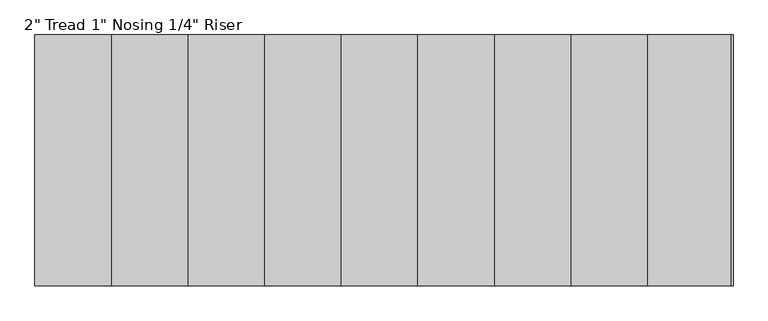
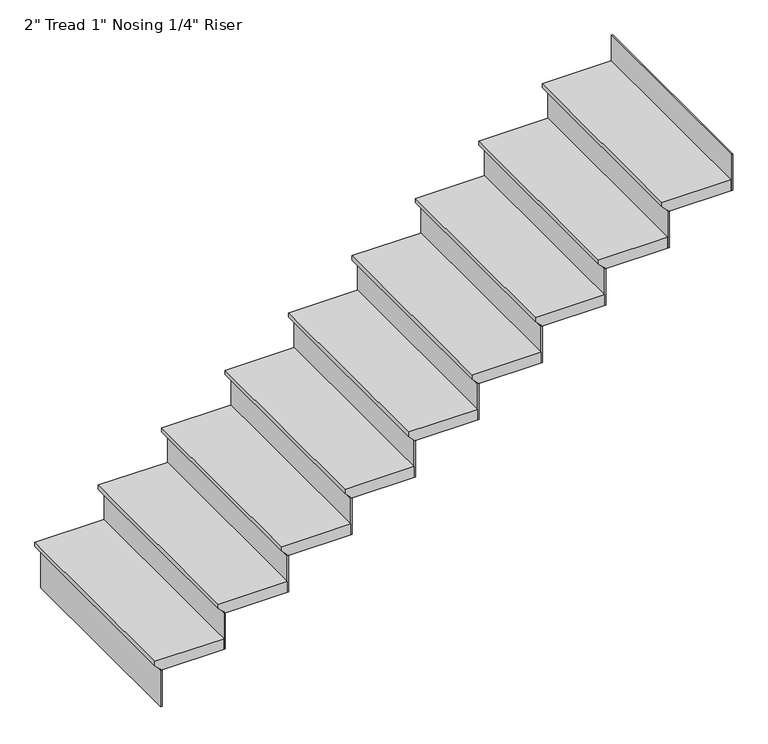
"""IFC4 building model written with IfcOpenShell, lengths in millimetres: stair flight geometry."""

from ifc_helpers import new_model, si_unit, frame, origin, place, context, project, spatial, polyline, outline, extrude, source, transform, mapped, element, save


def stair_flight_c7e5c723(model_context):
    return source(origin(), model_context, "Body", "SweptSolid", [
        extrude(outline(polyline([(4876.8, -14271.1777023), (4876.8, -14575.9777023), (4857.75, -14575.9777023), (4832.35, -14550.5777023), (4826.0, -14550.5777023), (4826.0, -14271.1777023), (4876.8, -14271.1777023)])), frame((0.0, 788.0679075, 0.0), z_axis=(0.0, 1.0, 0.0), x_axis=(0.0, 0.0, 1.0)), (0.0, 0.0, 1.0), 914.4),
        extrude(outline(polyline([(-14544.2277023, 788.0679075), (-14550.5777023, 788.0679075), (-14550.5777023, 1702.4679075), (-14544.2277023, 1702.4679075), (-14544.2277023, 788.0679075)])), frame((0.0, 0.0, 4656.6666667), z_axis=(0.0, 0.0, 1.0), x_axis=(1.0, 0.0, 0.0)), (0.0, 0.0, 1.0), 169.3333333),
        extrude(outline(polyline([(-14264.8277023, 788.0679075), (-14271.1777023, 788.0679075), (-14271.1777023, 1702.4679075), (-14264.8277023, 1702.4679075), (-14264.8277023, 788.0679075)])), frame((0.0, 0.0, 4826.0), z_axis=(0.0, 0.0, 1.0), x_axis=(1.0, 0.0, 0.0)), (0.0, 0.0, 1.0), 169.3333333),
        extrude(outline(polyline([(5046.1333333, -13991.7777023), (5046.1333333, -14296.5777023), (5027.0833333, -14296.5777023), (5001.6833333, -14271.1777023), (4995.3333333, -14271.1777023), (4995.3333333, -13991.7777023), (5046.1333333, -13991.7777023)])), frame((0.0, 788.0679075, 0.0), z_axis=(0.0, 1.0, 0.0), x_axis=(0.0, 0.0, 1.0)), (0.0, 0.0, 1.0), 914.4),
        extrude(outline(polyline([(-13985.4277023, 788.0679075), (-13991.7777023, 788.0679075), (-13991.7777023, 1702.4679075), (-13985.4277023, 1702.4679075), (-13985.4277023, 788.0679075)])), frame((0.0, 0.0, 4995.3333333), z_axis=(0.0, 0.0, 1.0), x_axis=(1.0, 0.0, 0.0)), (0.0, 0.0, 1.0), 169.3333333),
        extrude(outline(polyline([(5215.4666667, -13712.3777023), (5215.4666667, -14017.1777023), (5196.4166667, -14017.1777023), (5171.0166667, -13991.7777023), (5164.6666667, -13991.7777023), (5164.6666667, -13712.3777023), (5215.4666667, -13712.3777023)])), frame((0.0, 788.0679075, 0.0), z_axis=(0.0, 1.0, 0.0), x_axis=(0.0, 0.0, 1.0)), (0.0, 0.0, 1.0), 914.4),
        extrude(outline(polyline([(-13706.0277023, 788.0679075), (-13712.3777023, 788.0679075), (-13712.3777023, 1702.4679075), (-13706.0277023, 1702.4679075), (-13706.0277023, 788.0679075)])), frame((0.0, 0.0, 5164.6666667), z_axis=(0.0, 0.0, 1.0), x_axis=(1.0, 0.0, 0.0)), (0.0, 0.0, 1.0), 169.3333333),
        extrude(outline(polyline([(5384.8, -13432.9777023), (5384.8, -13737.7777023), (5365.75, -13737.7777023), (5340.35, -13712.3777023), (5334.0, -13712.3777023), (5334.0, -13432.9777023), (5384.8, -13432.9777023)])), frame((0.0, 788.0679075, 0.0), z_axis=(0.0, 1.0, 0.0), x_axis=(0.0, 0.0, 1.0)), (0.0, 0.0, 1.0), 914.4),
        extrude(outline(polyline([(-13426.6277023, 788.0679075), (-13432.9777023, 788.0679075), (-13432.9777023, 1702.4679075), (-13426.6277023, 1702.4679075), (-13426.6277023, 788.0679075)])), frame((0.0, 0.0, 5334.0), z_axis=(0.0, 0.0, 1.0), x_axis=(1.0, 0.0, 0.0)), (0.0, 0.0, 1.0), 169.3333333),
        extrude(outline(polyline([(5554.1333333, -13153.5777023), (5554.1333333, -13458.3777023), (5535.0833333, -13458.3777023), (5509.6833333, -13432.9777023), (5503.3333333, -13432.9777023), (5503.3333333, -13153.5777023), (5554.1333333, -13153.5777023)])), frame((0.0, 788.0679075, 0.0), z_axis=(0.0, 1.0, 0.0), x_axis=(0.0, 0.0, 1.0)), (0.0, 0.0, 1.0), 914.4),
        extrude(outline(polyline([(-13147.2277023, 788.0679075), (-13153.5777023, 788.0679075), (-13153.5777023, 1702.4679075), (-13147.2277023, 1702.4679075), (-13147.2277023, 788.0679075)])), frame((0.0, 0.0, 5503.3333333), z_axis=(0.0, 0.0, 1.0), x_axis=(1.0, 0.0, 0.0)), (0.0, 0.0, 1.0), 169.3333333),
        extrude(outline(polyline([(5723.4666667, -12874.1777023), (5723.4666667, -13178.9777023), (5704.4166667, -13178.9777023), (5679.0166667, -13153.5777023), (5672.6666667, -13153.5777023), (5672.6666667, -12874.1777023), (5723.4666667, -12874.1777023)])), frame((0.0, 788.0679075, 0.0), z_axis=(0.0, 1.0, 0.0), x_axis=(0.0, 0.0, 1.0)), (0.0, 0.0, 1.0), 914.4),
        extrude(outline(polyline([(-12867.8277023, 788.0679075), (-12874.1777023, 788.0679075), (-12874.1777023, 1702.4679075), (-12867.8277023, 1702.4679075), (-12867.8277023, 788.0679075)])), frame((0.0, 0.0, 5672.6666667), z_axis=(0.0, 0.0, 1.0), x_axis=(1.0, 0.0, 0.0)), (0.0, 0.0, 1.0), 169.3333333),
        extrude(outline(polyline([(5892.8, -12594.7777023), (5892.8, -12899.5777023), (5873.75, -12899.5777023), (5848.35, -12874.1777023), (5842.0, -12874.1777023), (5842.0, -12594.7777023), (5892.8, -12594.7777023)])), frame((0.0, 788.0679075, 0.0), z_axis=(0.0, 1.0, 0.0), x_axis=(0.0, 0.0, 1.0)), (0.0, 0.0, 1.0), 914.4),
        extrude(outline(polyline([(-12588.4277023, 788.0679075), (-12594.7777023, 788.0679075), (-12594.7777023, 1702.4679075), (-12588.4277023, 1702.4679075), (-12588.4277023, 788.0679075)])), frame((0.0, 0.0, 5842.0), z_axis=(0.0, 0.0, 1.0), x_axis=(1.0, 0.0, 0.0)), (0.0, 0.0, 1.0), 169.3333333),
        extrude(outline(polyline([(6062.1333333, -12315.3777023), (6062.1333333, -12620.1777023), (6043.0833333, -12620.1777023), (6017.6833333, -12594.7777023), (6011.3333333, -12594.7777023), (6011.3333333, -12315.3777023), (6062.1333333, -12315.3777023)])), frame((0.0, 788.0679075, 0.0), z_axis=(0.0, 1.0, 0.0), x_axis=(0.0, 0.0, 1.0)), (0.0, 0.0, 1.0), 914.4),
        extrude(outline(polyline([(-12309.0277023, 788.0679075), (-12315.3777023, 788.0679075), (-12315.3777023, 1702.4679075), (-12309.0277023, 1702.4679075), (-12309.0277023, 788.0679075)])), frame((0.0, 0.0, 6011.3333333), z_axis=(0.0, 0.0, 1.0), x_axis=(1.0, 0.0, 0.0)), (0.0, 0.0, 1.0), 169.3333333),
        extrude(outline(polyline([(-12029.6277023, 788.0679075), (-12035.9777023, 788.0679075), (-12035.9777023, 1702.4679075), (-12029.6277023, 1702.4679075), (-12029.6277023, 788.0679075)])), frame((0.0, 0.0, 6180.6666667), z_axis=(0.0, 0.0, 1.0), x_axis=(1.0, 0.0, 0.0)), (0.0, 0.0, 1.0), 169.3333333),
        extrude(outline(polyline([(6231.4666667, -12035.9777023), (6231.4666667, -12340.7777023), (6212.4166667, -12340.7777023), (6187.0166667, -12315.3777023), (6180.6666667, -12315.3777023), (6180.6666667, -12035.9777023), (6231.4666667, -12035.9777023)])), frame((0.0, 788.0679075, 0.0), z_axis=(0.0, 1.0, 0.0), x_axis=(0.0, 0.0, 1.0)), (0.0, 0.0, 1.0), 914.4),
    ])


if __name__ == "__main__":
    model = new_model("IFC4")
    model_context = context("Model", 3, world=origin())
    ifc_project = project(units=[si_unit("LENGTHUNIT", "METRE", prefix="MILLI")], contexts=[model_context])
    site = spatial("IfcSite", under=ifc_project)
    building = spatial("IfcBuilding", under=site)
    placement = place(None, origin())
    stair_flight_shape = stair_flight_c7e5c723(model_context)
    element("IfcStairFlight", 1, ObjectType="2\" Tread 1\" Nosing 1/4\" Riser", at=placement, inside=building, context=model_context, shape_type="MappedRepresentation", body=[
        mapped(stair_flight_shape, transform((0.0, 0.0, 0.0), x_axis=(1.0, 0.0, 0.0), y_axis=(0.0, 1.0, 0.0), z_axis=(0.0, 0.0, 1.0))),
    ])
    save(model, "model.ifc")
